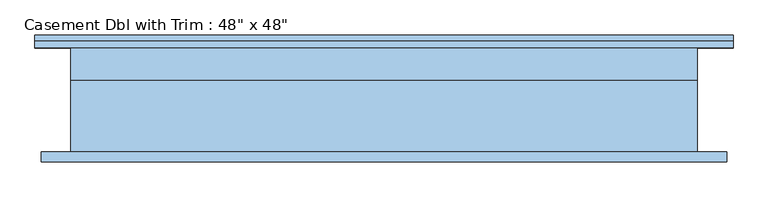
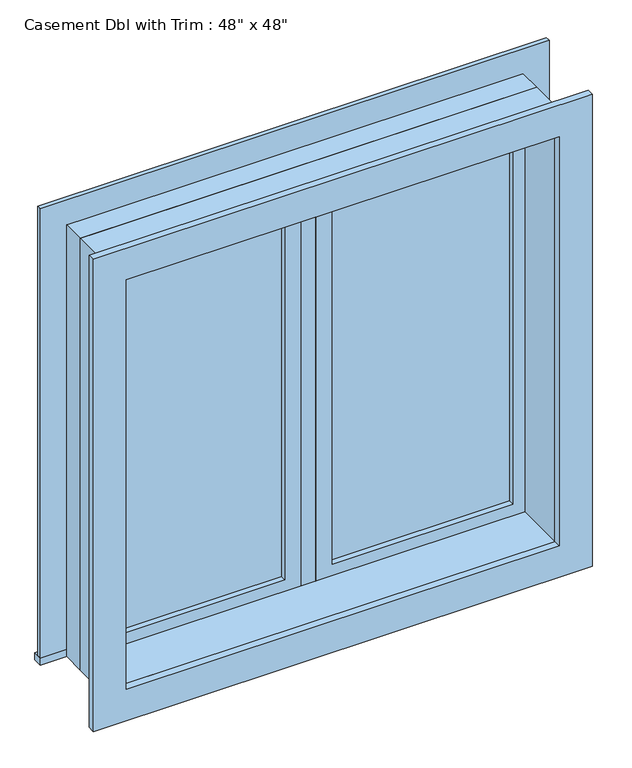
"""IFC4 building model written with IfcOpenShell, lengths in millimetres: window geometry."""

from ifc_helpers import new_model, si_unit, frame, origin, place, context, project, spatial, polyline, outline, extrude, source, transform, mapped, element, save


def window_0862ab64(model_context):
    return source(origin(), model_context, "Body", "SweptSolid", [
        extrude(outline(polyline([(63.5, 85.725), (546.1, 85.725), (546.1, 73.025), (63.5, 73.025), (63.5, 85.725)])), frame((0.0, 0.0, 977.9), z_axis=(0.0, 0.0, 1.0), x_axis=(1.0, 0.0, 0.0)), (0.0, 0.0, 1.0), 1092.2),
        extrude(outline(polyline([(2114.55, 19.05), (933.45, 19.05), (933.45, 590.55), (2114.55, 590.55), (2114.55, 19.05)]), holes=[polyline([(2070.1, 63.5), (2070.1, 546.1), (977.9, 546.1), (977.9, 63.5), (2070.1, 63.5)])]), frame((0.0, 57.15, 0.0), z_axis=(0.0, 1.0, 0.0), x_axis=(0.0, 0.0, 1.0)), (0.0, 0.0, 1.0), 44.45),
        extrude(outline(polyline([(19.05, 57.15), (-19.05, 57.15), (-19.05, 120.65), (19.05, 120.65), (19.05, 57.15)])), frame((0.0, 0.0, 933.45), z_axis=(0.0, 0.0, 1.0), x_axis=(1.0, 0.0, 0.0)), (0.0, 0.0, 1.0), 1181.1),
        extrude(outline(polyline([(-679.45, 146.05), (679.45, 146.05), (679.45, 120.65), (-679.45, 120.65), (-679.45, 146.05)])), frame((0.0, 0.0, 914.4), z_axis=(0.0, 0.0, 1.0), x_axis=(1.0, 0.0, 0.0)), (0.0, 0.0, 1.0), 19.05),
        extrude(outline(polyline([(2114.55, -590.55), (2114.55, 590.55), (933.45, 590.55), (933.45, 679.45), (2203.45, 679.45), (2203.45, -679.45), (933.45, -679.45), (933.45, -590.55), (2114.55, -590.55)])), frame((0.0, 120.65, 0.0), z_axis=(0.0, 1.0, 0.0), x_axis=(0.0, 0.0, 1.0)), (0.0, 0.0, 1.0), 12.7),
        extrude(outline(polyline([(2190.75, 666.75), (2190.75, -666.75), (857.25, -666.75), (857.25, 666.75), (2190.75, 666.75)]), holes=[polyline([(2101.85, 577.85), (946.15, 577.85), (946.15, -577.85), (2101.85, -577.85), (2101.85, 577.85)])]), frame((0.0, -101.6, 0.0), z_axis=(0.0, 1.0, 0.0), x_axis=(0.0, 0.0, 1.0)), (0.0, 0.0, 1.0), 19.05),
        extrude(outline(polyline([(-63.5, 73.025), (-546.1, 73.025), (-546.1, 85.725), (-63.5, 85.725), (-63.5, 73.025)])), frame((0.0, 0.0, 977.9), z_axis=(0.0, 0.0, 1.0), x_axis=(1.0, 0.0, 0.0)), (0.0, 0.0, 1.0), 1092.2),
        extrude(outline(polyline([(2114.55, -590.55), (933.45, -590.55), (933.45, -19.05), (2114.55, -19.05), (2114.55, -590.55)]), holes=[polyline([(2070.1, -546.1), (2070.1, -63.5), (977.9, -63.5), (977.9, -546.1), (2070.1, -546.1)])]), frame((0.0, 57.15, 0.0), z_axis=(0.0, 1.0, 0.0), x_axis=(0.0, 0.0, 1.0)), (0.0, 0.0, 1.0), 44.45),
        extrude(outline(polyline([(2133.6, -609.6), (914.4, -609.6), (914.4, 609.6), (2133.6, 609.6), (2133.6, -609.6)]), holes=[polyline([(2101.85, -577.85), (2101.85, 577.85), (946.15, 577.85), (946.15, -577.85), (2101.85, -577.85)])]), frame((0.0, -82.55, 0.0), z_axis=(0.0, 1.0, 0.0), x_axis=(0.0, 0.0, 1.0)), (0.0, 0.0, 1.0), 139.7),
        extrude(outline(polyline([(2133.6, 609.6), (2133.6, -609.6), (914.4, -609.6), (914.4, 609.6), (2133.6, 609.6)]), holes=[polyline([(2114.55, 590.55), (933.45, 590.55), (933.45, -590.55), (2114.55, -590.55), (2114.55, 590.55)])]), frame((0.0, 57.15, 0.0), z_axis=(0.0, 1.0, 0.0), x_axis=(0.0, 0.0, 1.0)), (0.0, 0.0, 1.0), 63.5),
    ])


if __name__ == "__main__":
    model = new_model("IFC4")
    model_context = context("Model", 3, world=origin())
    ifc_project = project(units=[si_unit("LENGTHUNIT", "METRE", prefix="MILLI")], contexts=[model_context])
    site = spatial("IfcSite", under=ifc_project)
    building = spatial("IfcBuilding", under=site)
    placement = place(None, origin())
    window_shape = window_0862ab64(model_context)
    element("IfcWindow", 1, ObjectType="Casement Dbl with Trim : 48\" x 48\"", at=placement, inside=building, context=model_context, shape_type="MappedRepresentation", body=[
        mapped(window_shape, transform((0.0, 0.0, 0.0), x_axis=(1.0, 0.0, 0.0), y_axis=(0.0, 1.0, 0.0), z_axis=(0.0, 0.0, 1.0))),
    ])
    save(model, "model.ifc")

# Revit data of these elements
# Type "Casement Dbl with Trim : 48\" x 48\""
#   Type Mark = "10"
#   Construction Type Id = "GSP4R"
#   Assembly Code = "B2020100"
#   Analytic Construction = "1/8 in Pilkington single glazing"
#   Visual Light Transmittance = 0.9
#   Solar Heat Gain Coefficient = 0.78
#   Heat Transfer Coefficient (U) = 3.6886 W/(m²·K)
#   Height = 4' - 0"
#   Default Sill Height = 3' - 0"
#   Trim Projection - Ext. = 0' - 0 1/2"
#   Trim Projection - Int. = 0' - 0 3/4"
#   Trim Width - Exterior = 0' - 3 1/2"
#   Trim Width - Interior = 0' - 3 1/2"
#   Width = 4' - 0"
#   Window Inset = 0' - 0 3/4"
#   Glass Pane Material = Glass
#   Sash Material = Sash
#   Trim Exterior Material = Trim
#   Trim Interior Material = Trim
#   Wall Closure = (empty or 0)
# Element 1 (IfcWindow, "Casement Dbl with Trim : 48\" x 48\"")
#   Materials on its faces: "Sash", "Trim", "Glass"
# Materials
#   "Glass": class "Glass", colour RGB 0 128 192, transparency 0.75, Description = "Soda Lime Glass", Cost = 0
#   "Sash": class "Wood", colour RGB 224 178 126, transparency 0
#   "Trim": class "Wood", colour RGB 224 178 126, transparency 0
